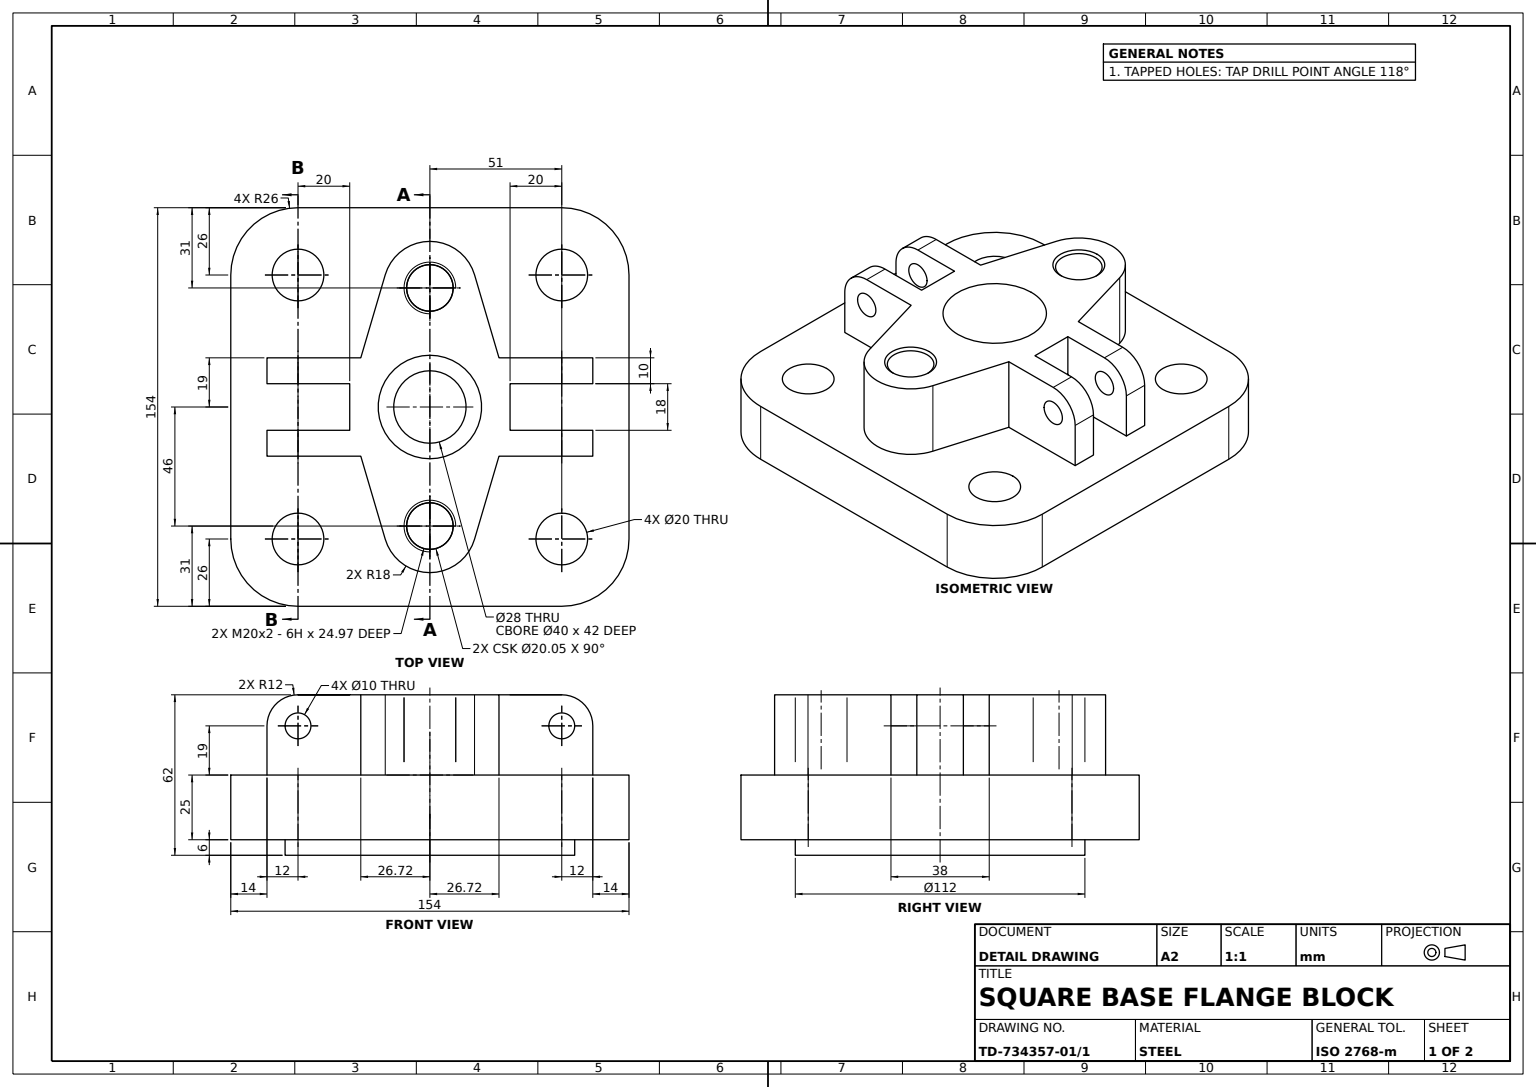
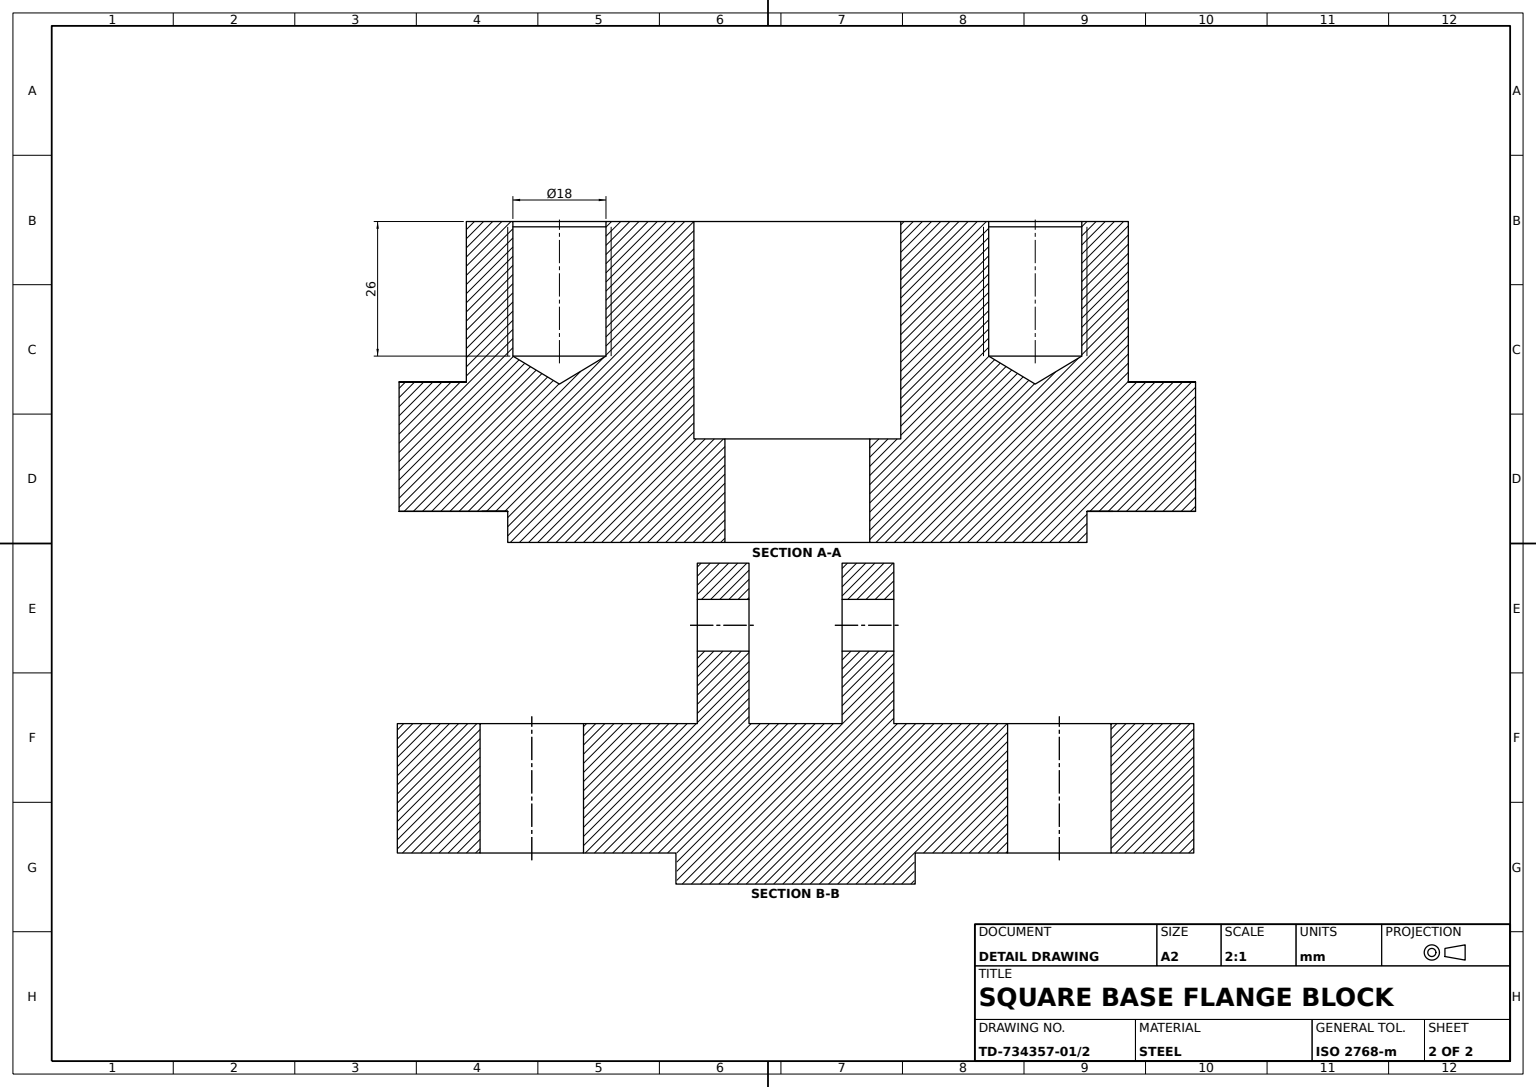
from build123d import *

# Parameters (mm, degrees)
BASE_PLATE_154X154X25_DEPTH      = 25
LOCATING_SPIGOT_SKETCH_112_R     = 56
LOCATING_SPIGOT_112X6_DEPTH      = 6
PIVOT_BOSS_WITH_LUGS_DEPTH       = 31
PIVOT_BOSS_FILLETS_R12_R         = 12
LUG_PIN_HOLES_SKETCH_10_R        = 5
LUG_PIN_HOLES_10_DEPTH           = 136.207248326
CENTRE_BORE_SKETCH_40_R          = 20
CENTRE_BORE_40_DEPTH             = 42
THROUGH_BORE_SKETCH_28_R         = 14
THROUGH_BORE_28_DEPTH            = 42
TAPPED_HOLES_M20X2_0_D           = 18
TAPPED_HOLES_M20X2_0_DEPTH       = 26
TAPPED_HOLES_M20X2_0_CSINK_D     = 20.05
TAPPED_HOLES_M20X2_0_CSINK_ANGLE = 90
TAPPED_HOLES_M20X2_0_TIP         = 5.407745571
MOUNTING_HOLES_SKETCH_4X_20_R    = 10
MOUNTING_HOLES_4X_20_DEPTH       = 42


with BuildPart() as part:
    # Base Plate Profile 154x154 R26 → Base Plate 154x154x25 (new body)
    with BuildSketch(Plane(origin=(0, 0, 0), x_dir=(1, 0, 0), z_dir=(0, 1, 0))):
        with BuildLine():
            Line((-51, -77), (51, -77))
            ThreePointArc((51, -77), (69.384776311, -69.384776311), (77, -51))
            Line((77, -51), (77, 51))
            ThreePointArc((77, 51), (69.384776311, 69.384776311), (51, 77))
            Line((51, 77), (-51, 77))
            ThreePointArc((-51, 77), (-69.384776311, 69.384776311), (-77, 51))
            Line((-77, 51), (-77, -51))
            ThreePointArc((-77, -51), (-69.384776311, -69.384776311), (-51, -77))
        make_face()
    extrude(amount=BASE_PLATE_154X154X25_DEPTH)

    # Locating Spigot Sketch Ø112 → Locating Spigot Ø112x6 (add)
    with BuildSketch(Plane.XZ):
        with Locations(Location((0, 0, 0), (0, 0, 270))):
            Circle(LOCATING_SPIGOT_SKETCH_112_R)
    extrude(amount=LOCATING_SPIGOT_112X6_DEPTH)

    # Pivot Boss Profile → Pivot Boss with Lugs (add)
    with BuildSketch(Plane(origin=(0, 25, 0), x_dir=(1, 0, 0), z_dir=(0, 1, 0))):
        with BuildLine():
            Line((-17.266235066, 51.086956522), (-26.719653956, 19))
            Line((-26.719653956, 19), (-63, 19))
            Line((-63, 19), (-63, 9))
            Line((-63, 9), (-31, 9))
            Line((-31, 9), (-31, -9))
            Line((-31, -9), (-63, -9))
            Line((-63, -9), (-63, -19))
            Line((-63, -19), (-26.719653956, -19))
            Line((-26.719653956, -19), (-17.266235066, -51.086956522))
            ThreePointArc((-17.266235066, -51.086956522), (0, -64), (17.266235066, -51.086956522))
            Line((17.266235066, -51.086956522), (26.719653956, -19))
            Line((26.719653956, -19), (63, -19))
            Line((63, -19), (63, -9))
            Line((63, -9), (31, -9))
            Line((31, -9), (31, 9))
            Line((31, 9), (63, 9))
            Line((63, 9), (63, 19))
            Line((63, 19), (26.719653956, 19))
            Line((26.719653956, 19), (17.266235066, 51.086956522))
            ThreePointArc((17.266235066, 51.086956522), (0, 64), (-17.266235066, 51.086956522))
        make_face()
    extrude(amount=PIVOT_BOSS_WITH_LUGS_DEPTH)

    # Pivot Boss Fillets R12
    pivot_boss_fillets_r12_edges = [part.edges().sort_by_distance(p)[0] for p in [
        (-63, 56, 14),
        (63, 56, 14),
        (63, 56, -14),
        (-63, 56, -14),
    ]]
    fillet(pivot_boss_fillets_r12_edges, radius=PIVOT_BOSS_FILLETS_R12_R)

    # Lug Pin Holes Sketch Ø10 → Lug Pin Holes Ø10 (cut, through all)
    with BuildSketch(Plane.XY.offset(19)):
        with Locations((-51, 44)):
            Circle(LUG_PIN_HOLES_SKETCH_10_R)
        with Locations((51, 44)):
            Circle(LUG_PIN_HOLES_SKETCH_10_R)
    extrude(amount=-LUG_PIN_HOLES_10_DEPTH, mode=Mode.SUBTRACT)

    # Centre Bore Sketch Ø40 → Centre Bore Ø40 (cut)
    with BuildSketch(Plane(origin=(0, 56, 0), x_dir=(1, 0, 0), z_dir=(0, 1, 0))):
        with Locations(Location((0, 0, 0), (0, 0, 270))):
            Circle(CENTRE_BORE_SKETCH_40_R)
    extrude(amount=-CENTRE_BORE_40_DEPTH, mode=Mode.SUBTRACT)

    # Through Bore Sketch Ø28 → Through Bore Ø28 (cut)
    with BuildSketch(Plane(origin=(0, 14, 0), x_dir=(1, 0, 0), z_dir=(0, 1, 0))):
        with Locations(Location((0, 0, 0), (0, 0, 270))):
            Circle(THROUGH_BORE_SKETCH_28_R)
    extrude(amount=-THROUGH_BORE_28_DEPTH, mode=Mode.SUBTRACT)

    # Tapped Holes M20x2.0
    with Locations(Plane(origin=(0, 56, 0), x_dir=(1, 0, 0), z_dir=(0, 1, 0))):
        with Locations((0, 46), (0, -46)):
            CounterSinkHole(TAPPED_HOLES_M20X2_0_D / 2, TAPPED_HOLES_M20X2_0_CSINK_D / 2, depth=TAPPED_HOLES_M20X2_0_DEPTH, counter_sink_angle=TAPPED_HOLES_M20X2_0_CSINK_ANGLE)
            with Locations((0, 0, -(TAPPED_HOLES_M20X2_0_DEPTH + TAPPED_HOLES_M20X2_0_TIP / 2))):  # 118° drill point
                Cone(0, TAPPED_HOLES_M20X2_0_D / 2, TAPPED_HOLES_M20X2_0_TIP, mode=Mode.SUBTRACT)

    # Mounting Holes Sketch 4xØ20 → Mounting Holes 4xØ20 (cut)
    with BuildSketch(Plane(origin=(0, 25, 0), x_dir=(1, 0, 0), z_dir=(0, 1, 0))):
        with Locations(Location((51, 51, 0), (0, 0, 270))):
            Circle(MOUNTING_HOLES_SKETCH_4X_20_R)
        with Locations(Location((-51, 51, 0), (0, 0, 270))):
            Circle(MOUNTING_HOLES_SKETCH_4X_20_R)
        with Locations(Location((-51, -51, 0), (0, 0, 270))):
            Circle(MOUNTING_HOLES_SKETCH_4X_20_R)
        with Locations(Location((51, -51, 0), (0, 0, 270))):
            Circle(MOUNTING_HOLES_SKETCH_4X_20_R)
    extrude(amount=-MOUNTING_HOLES_4X_20_DEPTH, mode=Mode.SUBTRACT)


solid = part.part
